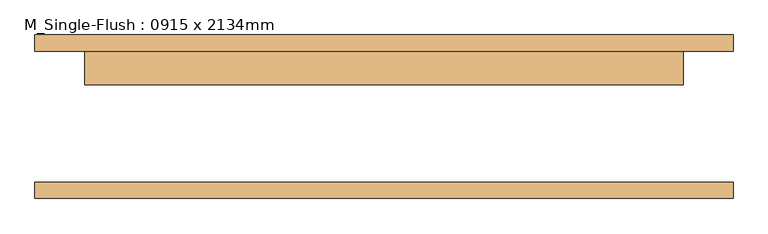
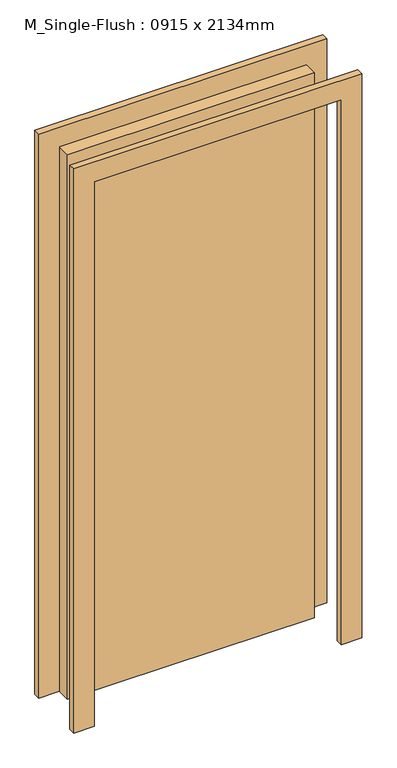
"""IFC4 building model written with IfcOpenShell, lengths in millimetres: door geometry, M_Single-Flush : 0915 x 2134mm."""

from ifc_helpers import new_model, si_unit, frame, origin, origin_with_axes, place, context, project, spatial, polyline, outline, extrude, source, transform, mapped, element, save


def m_single_flush_0915_x_2134mm_6a9e8738(model_context):
    return source(origin(), model_context, "Body", "SweptSolid", [
        extrude(outline(polyline([(2210.0, -533.5), (0.0, -533.5), (0.0, -457.5), (2134.0, -457.5), (2134.0, 457.5), (0.0, 457.5), (0.0, 533.5), (2210.0, 533.5), (2210.0, -533.5)])), frame((0.0, 100.0, 0.0), z_axis=(0.0, 1.0, 0.0), x_axis=(0.0, 0.0, 1.0)), (0.0, 0.0, 1.0), 25.0),
        extrude(outline(polyline([(2210.0, 533.5), (2210.0, -533.5), (0.0, -533.5), (0.0, -457.5), (2134.0, -457.5), (2134.0, 457.5), (0.0, 457.5), (0.0, 533.5), (2210.0, 533.5)])), frame((0.0, -125.0, 0.0), z_axis=(0.0, 1.0, 0.0), x_axis=(0.0, 0.0, 1.0)), (0.0, 0.0, 1.0), 25.0),
        extrude(outline(polyline([(457.5, 49.0), (-457.5, 49.0), (-457.5, 100.0), (457.5, 100.0), (457.5, 49.0)])), origin_with_axes(), (0.0, 0.0, 1.0), 2134.0),
    ])


if __name__ == "__main__":
    model = new_model("IFC4")
    model_context = context("Model", 3, world=origin())
    ifc_project = project(units=[si_unit("LENGTHUNIT", "METRE", prefix="MILLI")], contexts=[model_context])
    site = spatial("IfcSite", under=ifc_project)
    building = spatial("IfcBuilding", under=site)
    placement = place(None, origin())
    m_single_flush_0915_x_2134mm_shape = m_single_flush_0915_x_2134mm_6a9e8738(model_context)
    element("IfcDoor", 1, ObjectType="M_Single-Flush : 0915 x 2134mm", at=placement, inside=building, context=model_context, shape_type="MappedRepresentation", body=[
        mapped(m_single_flush_0915_x_2134mm_shape, transform((0.0, 0.0, 0.0), x_axis=(1.0, 0.0, 0.0), y_axis=(0.0, 1.0, 0.0), z_axis=(0.0, 0.0, 1.0))),
    ])
    save(model, "model.ifc")

# Revit data of these elements
# Type "M_Single-Flush : 0915 x 2134mm"
#   Type Mark = "15"
#   Thickness = 51 mm
#   Height = 2134 mm
#   Trim Projection Ext = 25 mm
#   Trim Projection Int = 25 mm
#   Trim Width = 76 mm
#   Width = 915 mm
#   Door Material = Door - Panel
#   Frame Material = Door - Frame
#   Function = (empty or 0)
#   Wall Closure = (empty or 0)
# Element 1 (IfcDoor, "M_Single-Flush : 0915 x 2134mm")
#   Materials on its faces: "Door - Frame", "Door - Panel"
# Materials
#   "Door - Panel": class "Wood", colour RGB 114 82 51, transparency 0
#   "Door - Frame": colour RGB 153 76 43, transparency 0
